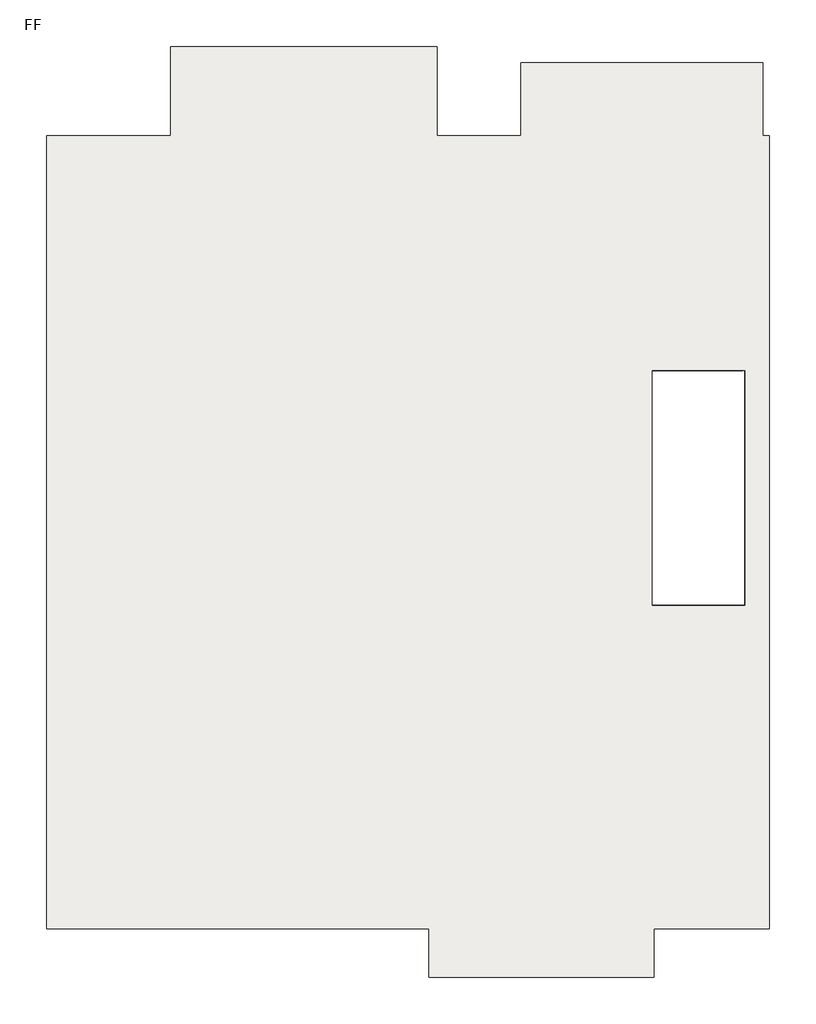
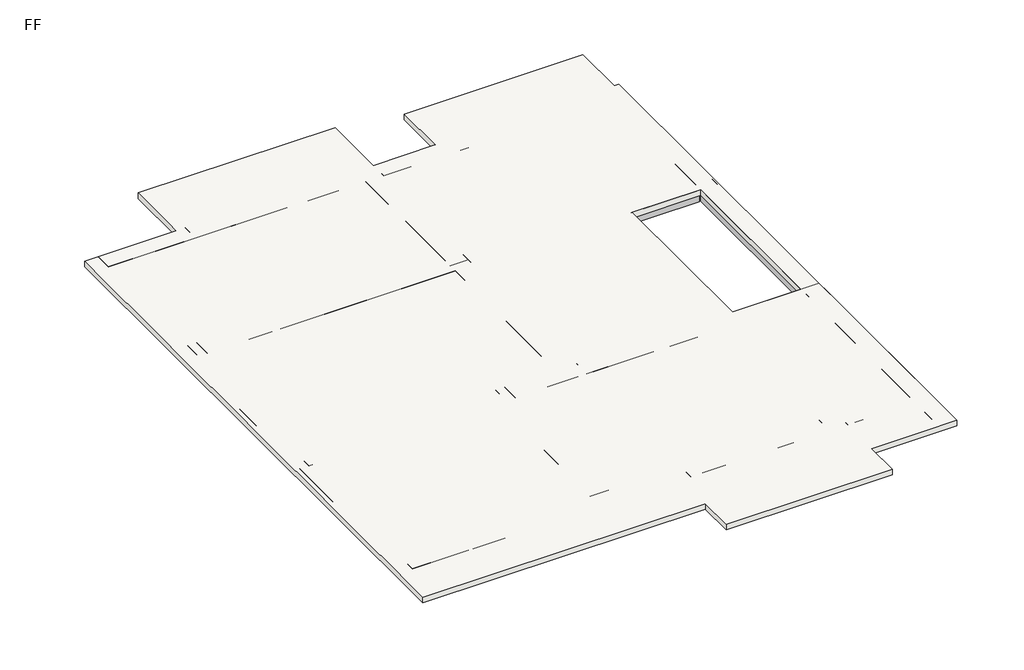
# One storey: 17 beams, 1 slab.
"""IFC4 building model written with IfcOpenShell, lengths in millimetres."""

from ifc_helpers import new_model, si_unit, frame, origin, place, context, project, spatial, polyline, outline, extrude, faceted_brep, element, save

model = new_model("IFC4")

# Units and contexts
model_context = context("Model", 3, world=origin())
ifc_project = project(units=[si_unit("LENGTHUNIT", "METRE", prefix="MILLI")], contexts=[model_context])

# Site, building, storey
site = spatial("IfcSite", under=ifc_project)
building = spatial("IfcBuilding", under=site)
storey = spatial("IfcBuildingStorey", under=building, Name="FF", Elevation=3505.2)

# Beams
placement = place(None, origin())
element("IfcBeam", 1, ObjectType="Concrete-Rectangular Beam : 18X12", at=placement, inside=storey, context=model_context, shape_type="Brep", body=[
    faceted_brep([(5601.0916032, 10641.5241878, 3505.2), (5601.0916032, 10184.3241878, 3505.2), (12153.8099466, 10184.3241878, 3505.2), (12611.0099466, 10184.3241878, 3505.2), (12611.0099466, 10412.9241878, 3505.2), (12382.4099466, 10412.9241878, 3505.2), (12382.4099466, 10641.5241878, 3505.2), (7823.1099466, 10641.5241878, 3505.2), (7823.1099466, 10412.9241878, 3505.2), (7594.5099466, 10412.9241878, 3505.2), (7594.5099466, 10641.5241878, 3505.2), (5601.0916032, 10184.3241878, 3200.4), (12153.8099466, 10184.3241878, 3200.4), (12611.0099466, 10184.3241878, 3200.4), (5601.0916032, 10641.5241878, 3200.4), (7594.5099466, 10641.5241878, 3200.4), (7594.5099466, 10412.9241878, 3200.4), (7823.1099466, 10412.9241878, 3200.4), (7823.1099466, 10641.5241878, 3200.4), (12382.4099466, 10641.5241878, 3200.4), (12382.4099466, 10412.9241878, 3200.4), (12611.0099466, 10412.9241878, 3200.4)], [[[0, 1, 2, 3, 4, 5, 6, 7, 8, 9, 10]], [[1, 11, 12, 13, 3, 2]], [[11, 14, 15, 16, 17, 18, 19, 20, 21, 13, 12]], [[6, 19, 18, 7]], [[0, 14, 11, 1]], [[20, 5, 4, 21]], [[5, 20, 19, 6]], [[17, 8, 7, 18]], [[8, 17, 16, 9]], [[9, 16, 15, 10]], [[14, 0, 10, 15]], [[3, 13, 21, 4]]]),
])
element("IfcBeam", 2, ObjectType="Concrete-Rectangular Beam : 18X12", at=placement, inside=storey, context=model_context, shape_type="Brep", body=[
    faceted_brep([(18859.8916032, 10184.3241878, 3505.2), (18859.8916032, 10412.9241878, 3505.2), (18402.6916032, 10412.9241878, 3505.2), (18402.6916032, 10641.5241878, 3505.2), (12839.6099466, 10641.5241878, 3505.2), (12839.6099466, 10412.9241878, 3505.2), (12611.0099466, 10412.9241878, 3505.2), (12611.0099466, 10184.3241878, 3505.2), (18402.6916032, 10184.3241878, 3505.2), (18859.8916032, 10184.3241878, 3200.4), (12611.0099466, 10184.3241878, 3200.4), (18402.6916032, 10184.3241878, 3200.4), (18859.8916032, 10412.9241878, 3200.4), (12611.0099466, 10412.9241878, 3200.4), (12839.6099466, 10412.9241878, 3200.4), (12839.6099466, 10641.5241878, 3200.4), (18402.6916032, 10641.5241878, 3200.4), (18402.6916032, 10412.9241878, 3200.4)], [[[0, 1, 2, 3, 4, 5, 6, 7, 8]], [[9, 0, 8, 7, 10, 11]], [[12, 9, 11, 10, 13, 14, 15, 16, 17]], [[3, 16, 15, 4]], [[14, 5, 4, 15]], [[5, 14, 13, 6]], [[17, 2, 1, 12]], [[2, 17, 16, 3]], [[0, 9, 12, 1]], [[7, 6, 13, 10]]]),
])
element("IfcBeam", 3, ObjectType="Concrete-Rectangular Beam : 18X12", at=placement, inside=storey, context=model_context, shape_type="Brep", body=[
    faceted_brep([(18859.8916032, 10184.3241878, 3505.2), (18402.6916032, 10184.3241878, 3505.2), (18402.6916032, 6450.5241878, 3505.2), (18823.689508, 6450.5241878, 3505.2), (18823.689508, 6221.9241878, 3505.2), (18402.6916032, 6221.9241878, 3505.2), (18402.6916032, 1802.3241878, 3505.2), (18859.8916032, 1802.3241878, 3505.2), (18402.6916032, 10184.3241878, 3200.4), (18402.6916032, 6450.5241878, 3200.4), (18859.8916032, 10184.3241878, 3200.4), (18859.8916032, 1802.3241878, 3200.4), (18402.6916032, 1802.3241878, 3200.4), (18402.6916032, 6221.9241878, 3200.4), (18823.689508, 6221.9241878, 3200.4), (18823.689508, 6450.5241878, 3200.4)], [[[0, 1, 2, 3, 4, 5, 6, 7]], [[1, 8, 9, 2]], [[8, 10, 11, 12, 13, 14, 15, 9]], [[10, 0, 7, 11]], [[1, 0, 10, 8]], [[15, 3, 2, 9]], [[3, 15, 14, 4]], [[4, 14, 13, 5]], [[7, 6, 12, 11]], [[5, 13, 12, 6]]]),
    faceted_brep([(18859.8916032, -4052.3758122, 3505.2), (18402.6916032, -4052.3758122, 3505.2), (18402.6916032, -4052.3758122, 3200.4), (18859.8916032, -4052.3758122, 3200.4), (18402.6916032, -3226.8758122, 3505.2), (18402.6916032, -2769.6758122, 3505.2), (18402.6916032, 1345.1241878, 3505.2), (18402.6916032, 1573.7241878, 3505.2), (18402.6916032, 1573.7241878, 3200.4), (18402.6916032, 1345.1241878, 3200.4), (18402.6916032, -2769.6758122, 3200.4), (18402.6916032, -3226.8758122, 3200.4), (18859.8916032, 1573.7241878, 3505.2), (18859.8916032, 1573.7241878, 3200.4)], [[[0, 1, 2, 3]], [[2, 1, 4, 5, 6, 7, 8, 9, 10, 11]], [[7, 12, 13, 8]], [[1, 0, 12, 7, 6, 5, 4]], [[3, 2, 11, 10, 9, 8, 13]], [[0, 3, 13, 12]]]),
])
element("IfcBeam", 4, ObjectType="Concrete-Rectangular Beam : 18X12", at=placement, inside=storey, context=model_context, shape_type="SweptSolid", body=[
    extrude(outline(polyline([(16230.9916032, -2998.2758122), (16230.9916032, -2769.6758122), (18402.6916032, -2769.6758122), (18402.6916032, -3226.8758122), (16688.1916032, -3226.8758122), (16688.1916032, -2998.2758122), (16230.9916032, -2998.2758122)])), frame((0.0, 0.0, 3200.4), z_axis=(0.0, 0.0, 1.0), x_axis=(1.0, 0.0, 0.0)), (0.0, 0.0, 1.0), 304.8),
])
element("IfcBeam", 5, ObjectType="Concrete-Rectangular Beam : 18X12", at=placement, inside=storey, context=model_context, shape_type="Brep", body=[
    faceted_brep([(16230.9916032, -3226.8758122, 3505.2), (16230.9916032, -2998.2758122, 3505.2), (16230.9916032, -2769.6758122, 3505.2), (12687.6916032, -2769.6758122, 3505.2), (12687.6916032, -3226.8758122, 3505.2), (16230.9916032, -3226.8758122, 3200.4), (12687.6916032, -3226.8758122, 3200.4), (16230.9916032, -2769.6758122, 3200.4), (16230.9916032, -2998.2758122, 3200.4), (12687.6916032, -2769.6758122, 3200.4)], [[[0, 1, 2, 3, 4]], [[5, 0, 4, 6]], [[7, 8, 5, 6, 9]], [[2, 7, 9, 3]], [[3, 9, 6, 4]], [[2, 1, 0, 5, 8, 7]]]),
])
element("IfcBeam", 6, ObjectType="Concrete-Rectangular Beam : 18X12", at=placement, inside=storey, context=model_context, shape_type="Brep", body=[
    faceted_brep([(12459.0916032, -3226.8758122, 3505.2), (12459.0916032, -2998.2758122, 3505.2), (12459.0916032, -2769.6758122, 3505.2), (10858.8916032, -2769.6758122, 3505.2), (10630.2916032, -2769.6758122, 3505.2), (10630.2916032, -3226.8758122, 3505.2), (12459.0916032, -2769.6758122, 3200.4), (10858.8916032, -2769.6758122, 3200.4), (10630.2916032, -2769.6758122, 3200.4), (12459.0916032, -2998.2758122, 3200.4), (12459.0916032, -3226.8758122, 3200.4), (10630.2916032, -3226.8758122, 3200.4), (10630.2916032, -2998.2758122, 3200.4)], [[[0, 1, 2, 3, 4, 5]], [[2, 6, 7, 8, 4, 3]], [[6, 9, 10, 11, 12, 8, 7]], [[10, 0, 5, 11]], [[0, 10, 9, 6, 2, 1]], [[5, 4, 8, 12, 11]]]),
])
element("IfcBeam", 7, ObjectType="Concrete-Rectangular Beam : 18X12", at=placement, inside=storey, context=model_context, shape_type="Brep", body=[
    faceted_brep([(10401.6916032, -2769.6758122, 3505.2), (10630.2916032, -2769.6758122, 3505.2), (10858.8916032, -2769.6758122, 3505.2), (10858.8916032, 1345.1241878, 3505.2), (10858.8916032, 1802.3241878, 3505.2), (10630.2916032, 1802.3241878, 3505.2), (10630.2916032, 1345.1241878, 3505.2), (10401.6916032, 1345.1241878, 3505.2), (10858.8916032, -2769.6758122, 3200.4), (10858.8916032, 1345.1241878, 3200.4), (10858.8916032, 1802.3241878, 3200.4), (10630.2916032, -2769.6758122, 3200.4), (10401.6916032, -2769.6758122, 3200.4), (10401.6916032, 1345.1241878, 3200.4), (10630.2916032, 1345.1241878, 3200.4), (10630.2916032, 1802.3241878, 3200.4)], [[[0, 1, 2, 3, 4, 5, 6, 7]], [[2, 8, 9, 10, 4, 3]], [[8, 11, 12, 13, 14, 15, 10, 9]], [[12, 0, 7, 13]], [[2, 1, 0, 12, 11, 8]], [[14, 6, 5, 15]], [[6, 14, 13, 7]], [[4, 10, 15, 5]]]),
])
element("IfcBeam", 8, ObjectType="Concrete-Rectangular Beam : 18X12", at=placement, inside=storey, context=model_context, shape_type="Brep", body=[
    faceted_brep([(12459.0916032, 1345.1241878, 3505.2), (12459.0916032, 1802.3241878, 3505.2), (12153.8099466, 1802.3241878, 3505.2), (10858.8916032, 1802.3241878, 3505.2), (10858.8916032, 1345.1241878, 3505.2), (12459.0916032, 1345.1241878, 3200.4), (10858.8916032, 1345.1241878, 3200.4), (12459.0916032, 1802.3241878, 3200.4), (10858.8916032, 1802.3241878, 3200.4), (12153.8099466, 1802.3241878, 3200.4)], [[[0, 1, 2, 3, 4]], [[5, 0, 4, 6]], [[7, 5, 6, 8, 9]], [[1, 7, 9, 8, 3, 2]], [[1, 0, 5, 7]], [[4, 3, 8, 6]]]),
])
element("IfcBeam", 9, ObjectType="Concrete-Rectangular Beam : 18X12", at=placement, inside=storey, context=model_context, shape_type="Brep", body=[
    faceted_brep([(18402.6916032, 1345.1241878, 3505.2), (18402.6916032, 1573.7241878, 3505.2), (18402.6916032, 1802.3241878, 3505.2), (12687.6916032, 1802.3241878, 3505.2), (12687.6916032, 1345.1241878, 3505.2), (18402.6916032, 1345.1241878, 3200.4), (12687.6916032, 1345.1241878, 3200.4), (18402.6916032, 1802.3241878, 3200.4), (18402.6916032, 1573.7241878, 3200.4), (12687.6916032, 1802.3241878, 3200.4)], [[[0, 1, 2, 3, 4]], [[5, 0, 4, 6]], [[7, 8, 5, 6, 9]], [[2, 7, 9, 3]], [[3, 9, 6, 4]], [[2, 1, 0, 5, 8, 7]]]),
])
element("IfcBeam", 10, ObjectType="Concrete-Rectangular Beam : 18X12", at=placement, inside=storey, context=model_context, shape_type="Brep", body=[
    faceted_brep([(5601.0916032, 1802.3241878, 3505.2), (5601.0916032, 1345.1241878, 3505.2), (5829.6916032, 1345.1241878, 3505.2), (10401.6916032, 1345.1241878, 3505.2), (10401.6916032, 1802.3241878, 3505.2), (5829.6916032, 1802.3241878, 3505.2), (5601.0916032, 1345.1241878, 3200.4), (5829.6916032, 1345.1241878, 3200.4), (10401.6916032, 1345.1241878, 3200.4), (5601.0916032, 1802.3241878, 3200.4), (5829.6916032, 1802.3241878, 3200.4), (10401.6916032, 1802.3241878, 3200.4)], [[[0, 1, 2, 3, 4, 5]], [[1, 6, 7, 8, 3, 2]], [[6, 9, 10, 11, 8, 7]], [[9, 0, 5, 4, 11, 10]], [[1, 0, 9, 6]], [[4, 3, 8, 11]]]),
])
element("IfcBeam", 11, ObjectType="Concrete-Rectangular Beam : 18X12", at=placement, inside=storey, context=model_context, shape_type="Brep", body=[
    faceted_brep([(5601.0916032, -2769.6758122, 3505.2), (5601.0916032, -3226.8758122, 3505.2), (10401.6916032, -3226.8758122, 3505.2), (10401.6916032, -2769.6758122, 3505.2), (5829.6916032, -2769.6758122, 3505.2), (5601.0916032, -3226.8758122, 3200.4), (10401.6916032, -3226.8758122, 3200.4), (5601.0916032, -2769.6758122, 3200.4), (5829.6916032, -2769.6758122, 3200.4), (10401.6916032, -2769.6758122, 3200.4)], [[[0, 1, 2, 3, 4]], [[1, 5, 6, 2]], [[5, 7, 8, 9, 6]], [[7, 0, 4, 3, 9, 8]], [[1, 0, 7, 5]], [[3, 2, 6, 9]]]),
])
element("IfcBeam", 12, ObjectType="Concrete-Rectangular Beam : 18X12", at=placement, inside=storey, context=model_context, shape_type="Brep", body=[
    faceted_brep([(5829.6916032, 1345.1241878, 3505.2), (5601.0916032, 1345.1241878, 3505.2), (5372.4916032, 1345.1241878, 3505.2), (5372.4916032, -2769.6758122, 3505.2), (5601.0916032, -2769.6758122, 3505.2), (5829.6916032, -2769.6758122, 3505.2), (5829.6916032, 1345.1241878, 3200.4), (5829.6916032, -2769.6758122, 3200.4), (5372.4916032, 1345.1241878, 3200.4), (5601.0916032, 1345.1241878, 3200.4), (5601.0916032, -2769.6758122, 3200.4), (5372.4916032, -2769.6758122, 3200.4)], [[[0, 1, 2, 3, 4, 5]], [[6, 0, 5, 7]], [[8, 9, 6, 7, 10, 11]], [[2, 8, 11, 3]], [[2, 1, 0, 6, 9, 8]], [[5, 4, 3, 11, 10, 7]]]),
])
element("IfcBeam", 13, ObjectType="Concrete-Rectangular Beam : 18X12", at=placement, inside=storey, context=model_context, shape_type="Brep", body=[
    faceted_brep([(5829.6916032, 6679.1241878, 3505.2), (5601.0916032, 6679.1241878, 3505.2), (5601.0916032, 6221.9241878, 3505.2), (5372.4916032, 6221.9241878, 3505.2), (5372.4916032, 1802.3241878, 3505.2), (5601.0916032, 1802.3241878, 3505.2), (5829.6916032, 1802.3241878, 3505.2), (5829.6916032, 6221.9241878, 3505.2), (5372.4916032, 6221.9241878, 3200.4), (5372.4916032, 1802.3241878, 3200.4), (5601.0916032, 6679.1241878, 3200.4), (5829.6916032, 6679.1241878, 3200.4), (5829.6916032, 6221.9241878, 3200.4), (5829.6916032, 1802.3241878, 3200.4), (5601.0916032, 1802.3241878, 3200.4), (5601.0916032, 6221.9241878, 3200.4)], [[[0, 1, 2, 3, 4, 5, 6, 7]], [[3, 8, 9, 4]], [[10, 11, 12, 13, 14, 9, 8, 15]], [[11, 0, 7, 6, 13, 12]], [[15, 2, 1, 10]], [[2, 15, 8, 3]], [[6, 5, 4, 9, 14, 13]], [[0, 11, 10, 1]]]),
])
element("IfcBeam", 14, ObjectType="Concrete-Rectangular Beam : 18X12", at=placement, inside=storey, context=model_context, shape_type="Brep", body=[
    faceted_brep([(5829.6916032, 6679.1241878, 3505.2), (5829.6916032, 6221.9241878, 3505.2), (7480.2099466, 6221.9241878, 3505.2), (7480.2099466, 6450.5241878, 3505.2), (7708.8099466, 6450.5241878, 3505.2), (7708.8099466, 6221.9241878, 3505.2), (12153.8099466, 6221.9241878, 3505.2), (12153.8099466, 6450.5241878, 3505.2), (12611.0099466, 6450.5241878, 3505.2), (12611.0099466, 6679.1241878, 3505.2), (12153.8099466, 6679.1241878, 3505.2), (12153.8099466, 6221.9241878, 3200.4), (7708.8099466, 6221.9241878, 3200.4), (5829.6916032, 6221.9241878, 3200.4), (5829.6916032, 6679.1241878, 3200.4), (12153.8099466, 6679.1241878, 3200.4), (12611.0099466, 6679.1241878, 3200.4), (12611.0099466, 6450.5241878, 3200.4), (12153.8099466, 6450.5241878, 3200.4), (7708.8099466, 6450.5241878, 3200.4), (7480.2099466, 6450.5241878, 3200.4), (7480.2099466, 6221.9241878, 3200.4)], [[[0, 1, 2, 3, 4, 5, 6, 7, 8, 9, 10]], [[11, 6, 5, 12]], [[13, 14, 15, 16, 17, 18, 11, 12, 19, 20, 21]], [[14, 0, 10, 9, 16, 15]], [[1, 0, 14, 13]], [[7, 18, 17, 8]], [[18, 7, 6, 11]], [[4, 19, 12, 5]], [[20, 3, 2, 21]], [[3, 20, 19, 4]], [[1, 13, 21, 2]], [[16, 9, 8, 17]]]),
])
element("IfcBeam", 15, ObjectType="Concrete-Rectangular Beam : 18X12", at=placement, inside=storey, context=model_context, shape_type="SweptSolid", body=[
    extrude(outline(polyline([(12153.8099466, 10184.3241878), (12611.0099466, 10184.3241878), (12611.0099466, 6679.1241878), (12153.8099466, 6679.1241878), (12153.8099466, 10184.3241878)])), frame((0.0, 0.0, 3200.4), z_axis=(0.0, 0.0, 1.0), x_axis=(1.0, 0.0, 0.0)), (0.0, 0.0, 1.0), 304.8),
])
element("IfcBeam", 16, ObjectType="Concrete-Rectangular Beam : 18X12", at=placement, inside=storey, context=model_context, shape_type="Brep", body=[
    faceted_brep([(18402.2099466, 6450.5241878, 3505.2), (18402.2099466, 6679.1241878, 3505.2), (12611.0099466, 6679.1241878, 3505.2), (12611.0099466, 6450.5241878, 3505.2), (12611.0099466, 6221.9241878, 3505.2), (18366.489508, 6221.9241878, 3505.2), (18366.489508, 6450.5241878, 3505.2), (18366.489508, 6221.9241878, 3200.4), (12611.0099466, 6221.9241878, 3200.4), (18402.2099466, 6679.1241878, 3200.4), (18402.2099466, 6450.5241878, 3200.4), (18366.489508, 6450.5241878, 3200.4), (12611.0099466, 6450.5241878, 3200.4), (12611.0099466, 6679.1241878, 3200.4)], [[[0, 1, 2, 3, 4, 5, 6]], [[7, 5, 4, 8]], [[9, 10, 11, 7, 8, 12, 13]], [[1, 9, 13, 2]], [[9, 1, 0, 10]], [[6, 11, 10, 0]], [[11, 6, 5, 7]], [[4, 3, 2, 13, 12, 8]]]),
])
element("IfcBeam", 17, ObjectType="Concrete-Rectangular Beam : 18X12", at=placement, inside=storey, context=model_context, shape_type="Brep", body=[
    faceted_brep([(12611.0099466, 6221.9241878, 3505.2), (12153.8099466, 6221.9241878, 3505.2), (12153.8099466, 1802.3241878, 3505.2), (12459.0916032, 1802.3241878, 3505.2), (12611.0099466, 1802.3241878, 3505.2), (12153.8099466, 6221.9241878, 3200.4), (12153.8099466, 1802.3241878, 3200.4), (12611.0099466, 6221.9241878, 3200.4), (12611.0099466, 1802.3241878, 3200.4), (12459.0916032, 1802.3241878, 3200.4)], [[[0, 1, 2, 3, 4]], [[1, 5, 6, 2]], [[5, 7, 8, 9, 6]], [[7, 0, 4, 8]], [[1, 0, 7, 5]], [[2, 6, 9, 8, 4, 3]]]),
])

# Slab
element("IfcSlab", 18, ObjectType="Concrete Slab - 6\"", at=placement, inside=storey, context=model_context, shape_type="SweptSolid", body=[
    extrude(outline(polyline([(7594.5099466, 10641.5241878), (7594.5099466, 12317.9241878), (12611.0099466, 12317.9241878), (12611.0099466, 10641.5241878), (14192.2689416, 10641.5241878), (14192.2689416, 12013.1241878), (18745.5916032, 12013.1241878), (18745.5916032, 10641.5241878), (18859.8916032, 10641.5241878), (18859.8916032, -4280.9758122), (16688.1916032, -4280.9758122), (16688.1916032, -5195.3758122), (12459.0916032, -5195.3758122), (12459.0916032, -4280.9758122), (5258.1916032, -4280.9758122), (5258.1916032, 10641.5241878), (7594.5099466, 10641.5241878)]), holes=[polyline([(18402.6916032, 6221.9241878), (16662.7916032, 6221.9241878), (16662.7916032, 1802.3241878), (18402.6916032, 1802.3241878), (18402.6916032, 6221.9241878)])]), frame((0.0, 0.0, 3352.8), z_axis=(0.0, 0.0, 1.0), x_axis=(1.0, 0.0, 0.0)), (0.0, 0.0, 1.0), 152.4),
])

save(model, "model.ifc")

# Revit data of these elements
# Type "Concrete-Rectangular Beam : 18X12"
#   Assembly Code = "B10"
#   Length [instance default] = 5' - 0"
#   b = 1' - 6"
#   h = 1' - 0"
#   Structural Material [instance default] = Concrete, Cast-in-Place gray
# Type "Concrete Slab - 6\""
#   Assembly Code = "B1010"
#   Function = 0
#   Layers, outside or top first: 0' - 6" "Concrete, Cast-in-Place gray" (function 1)
# Elements 1, 2, 3, 4, 5, 6, 7, 8, 9, 10, 11, 12, 13, 14, 15, 16, 17 (IfcBeam, "Concrete-Rectangular Beam : 18X12")
#   Structural Material = Concrete, Cast-in-Place gray
#   Phase Created = B10 - Superstructure
#   Materials on its faces: "Concrete, Cast-in-Place gray"
# Element 18 (IfcSlab, "Concrete Slab - 6\"")
#   Height Offset From Level = 0' - 0"
#   Phase Created = B10 - Superstructure
#   Materials on its faces: "Concrete, Cast-in-Place gray"
# Materials
#   "Concrete, Cast-in-Place gray": class "Concrete", colour RGB 192 192 192, transparency 0, Description = "Cast-in-place concrete", Cost = 0
